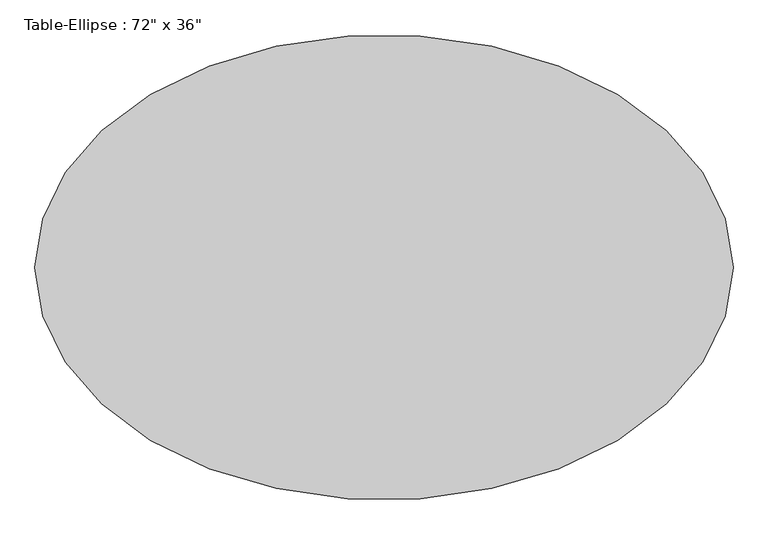
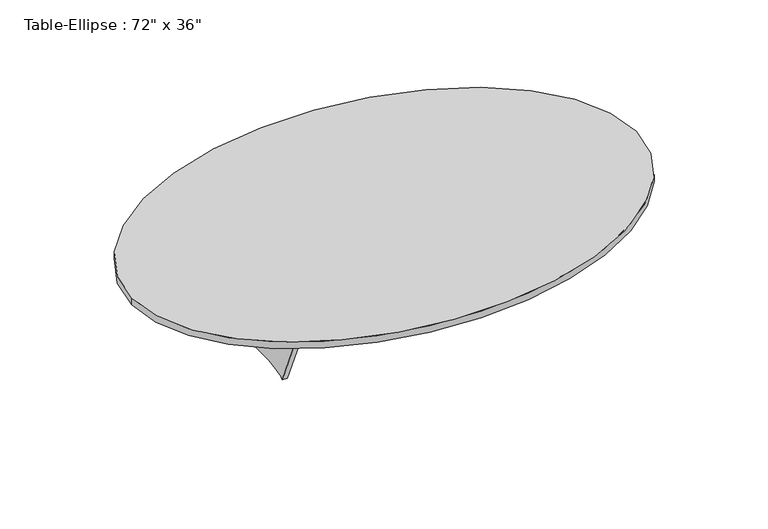
"""IFC4 building model written with IfcOpenShell, lengths in millimetres: furniture geometry."""

from ifc_helpers import new_model, si_unit, point, frame, origin, place, context, project, spatial, ellipse_curve, trimmed, source, transform, mapped, element, save
from ifc_brep_helpers import plane_surface, extruded_surface, advanced_brep


def furniture_1a6705e8(model_context):
    return source(origin(), model_context, "Body", "AdvancedBrep", [
        advanced_brep(
        [(-876.3, 19.05, 711.2), (876.3, 19.05, 711.2), (876.3, 19.05, 474.1333333), (-876.3, 19.05, 474.1333333), (-876.3, -19.05, 711.2), (-876.3, -19.05, 474.1333333), (876.3, -19.05, 474.1333333), (876.3, -19.05, 711.2)],
        [
            (0, 1),
            (1, 2),
            (2, 3, ellipse_curve(frame((0.0, 19.05, 474.1333333), z_axis=(0.0, -1.0, 0.0), x_axis=(1.0, 0.0, 0.0)), 876.3, 101.6)),
            (3, 0),
            (4, 5),
            (5, 6, ellipse_curve(frame((0.0, -19.05, 474.1333333), z_axis=(0.0, 1.0, 0.0), x_axis=(1.0, 0.0, 0.0)), 876.3, 101.6)),
            (6, 7),
            (7, 4),
            (0, 4),
            (7, 1),
            (6, 2),
            (5, 3),
        ],
        [
            plane_surface(frame((-876.3, 19.05, 711.2), z_axis=(0.0, 1.0, 0.0), x_axis=(1.0, 0.0, 0.0))),
            plane_surface(frame((-876.3, -19.05, 711.2), z_axis=(0.0, -1.0, 0.0), x_axis=(-1.0, 0.0, 0.0))),
            plane_surface(frame((-876.3, 19.05, 711.2), z_axis=(0.0, 0.0, 1.0), x_axis=(0.0, -1.0, 0.0))),
            plane_surface(frame((876.3, 19.05, 711.2), z_axis=(1.0, 0.0, 0.0), x_axis=(0.0, -1.0, 0.0))),
            extruded_surface(trimmed(ellipse_curve(frame((0.0, -57.15, 474.1333333), z_axis=(0.0, -1.0, 0.0), x_axis=(1.0, 0.0, 0.0)), 876.3, 101.6), [point((876.3, -57.15, 474.1333333))], [point((-876.3, -57.15, 474.1333333))], True, "CARTESIAN"), (0.0, 38.099999999999994, 0.0), 38.099999999999994),
            plane_surface(frame((-876.3, 19.05, 474.1333333), z_axis=(-1.0, 0.0, 0.0), x_axis=(0.0, -1.0, 0.0))),
        ],
        [
            (0, [[1, 2, 3, 4]]),
            (1, [[5, 6, 7, 8]]),
            (2, [[-1, 9, -8, 10]]),
            (3, [[-2, -10, -7, 11]]),
            (4, [[-3, -11, -6, 12]]),
            (5, [[-4, -12, -5, -9]]),
        ],
    ),
        advanced_brep(
        [(914.4, 609.6, 711.2), (914.4, -609.6, 711.2), (914.4, -304.8, 0.0), (914.4, 304.8, 0.0), (876.3, 609.6, 711.2), (876.3, 304.8, 0.0), (876.3, -304.8, 0.0), (876.3, -609.6, 711.2)],
        [
            (0, 1),
            (1, 2),
            (2, 3, ellipse_curve(frame((914.4, 0.0, 0.0), z_axis=(-1.0, 0.0, 0.0), x_axis=(0.0, 1.0, 0.0)), 304.8, 50.8)),
            (3, 0),
            (4, 5),
            (5, 6, ellipse_curve(frame((876.3, 0.0, 0.0), z_axis=(1.0, 0.0, 0.0), x_axis=(0.0, 1.0, 0.0)), 304.8, 50.8)),
            (6, 7),
            (7, 4),
            (0, 4),
            (7, 1),
            (6, 2),
            (5, 3),
        ],
        [
            plane_surface(frame((914.4, -609.6, 711.2), z_axis=(1.0, 0.0, 0.0), x_axis=(0.0, -1.0, 0.0))),
            plane_surface(frame((876.3, -609.6, 711.2), z_axis=(-1.0, 0.0, 0.0), x_axis=(0.0, 1.0, 0.0))),
            plane_surface(frame((914.4, 609.6, 711.2), z_axis=(0.0, 0.0, 1.0), x_axis=(-1.0, 0.0, 0.0))),
            plane_surface(frame((914.4, -609.6, 711.2), z_axis=(0.0, -0.919145030018057, -0.39391929857916985), x_axis=(-1.0, 0.0, 0.0))),
            extruded_surface(trimmed(ellipse_curve(frame((838.2, 0.0, 0.0), z_axis=(-1.0, 0.0, 0.0), x_axis=(0.0, 1.0, 0.0)), 304.8, 50.8), [point((838.2, -304.8, 0.0))], [point((838.2, 304.8, 0.0))], True, "CARTESIAN"), (38.09999999999991, 0.0, 0.0), 38.09999999999991),
            plane_surface(frame((914.4, 304.8, 0.0), z_axis=(0.0, 0.9191450300180644, -0.3939192985791526), x_axis=(-1.0, 0.0, 0.0))),
        ],
        [
            (0, [[1, 2, 3, 4]]),
            (1, [[5, 6, 7, 8]]),
            (2, [[-1, 9, -8, 10]]),
            (3, [[-2, -10, -7, 11]]),
            (4, [[-3, -11, -6, 12]]),
            (5, [[-4, -12, -5, -9]]),
        ],
    ),
        advanced_brep(
        [(-876.3, 609.6, 711.2), (-876.3, -609.6, 711.2), (-876.3, -304.8, 0.0), (-876.3, 304.8, 0.0), (-914.4, 609.6, 711.2), (-914.4, 304.8, 0.0), (-914.4, -304.8, 0.0), (-914.4, -609.6, 711.2)],
        [
            (0, 1),
            (1, 2),
            (2, 3, ellipse_curve(frame((-876.3, 0.0, 0.0), z_axis=(-1.0, 0.0, 0.0), x_axis=(0.0, 1.0, 0.0)), 304.8, 50.8)),
            (3, 0),
            (4, 5),
            (5, 6, ellipse_curve(frame((-914.4, 0.0, 0.0), z_axis=(1.0, 0.0, 0.0), x_axis=(0.0, 1.0, 0.0)), 304.8, 50.8)),
            (6, 7),
            (7, 4),
            (0, 4),
            (7, 1),
            (6, 2),
            (5, 3),
        ],
        [
            plane_surface(frame((-876.3, -609.6, 711.2), z_axis=(1.0, 0.0, 0.0), x_axis=(0.0, -1.0, 0.0))),
            plane_surface(frame((-914.4, -609.6, 711.2), z_axis=(-1.0, 0.0, 0.0), x_axis=(0.0, 1.0, 0.0))),
            plane_surface(frame((-876.3, 609.6, 711.2), z_axis=(0.0, 0.0, 1.0), x_axis=(-1.0, 0.0, 0.0))),
            plane_surface(frame((-876.3, -609.6, 711.2), z_axis=(0.0, -0.919145030018057, -0.3939192985791699), x_axis=(-1.0, 0.0, 0.0))),
            extruded_surface(trimmed(ellipse_curve(frame((-952.5, 0.0, 0.0), z_axis=(-1.0, 0.0, 0.0), x_axis=(0.0, 1.0, 0.0)), 304.8, 50.8), [point((-952.5, -304.8, 0.0))], [point((-952.5, 304.8, 0.0))], True, "CARTESIAN"), (38.10000000000002, 0.0, 0.0), 38.10000000000002),
            plane_surface(frame((-876.3, 304.8, 0.0), z_axis=(0.0, 0.9191450300180607, -0.3939192985791611), x_axis=(-1.0, 0.0, 0.0))),
        ],
        [
            (0, [[1, 2, 3, 4]]),
            (1, [[5, 6, 7, 8]]),
            (2, [[-1, 9, -8, 10]]),
            (3, [[-2, -10, -7, 11]]),
            (4, [[-3, -11, -6, 12]]),
            (5, [[-4, -12, -5, -9]]),
        ],
    ),
        advanced_brep(
        [(-1828.8, 0.0, 762.0), (1828.8, 0.0, 762.0), (-1828.8, 0.0, 711.2), (1828.8, 0.0, 711.2)],
        [
            (0, 1, ellipse_curve(frame((0.0, 0.0, 762.0), z_axis=(0.0, 0.0, 1.0), x_axis=(1.0, 0.0, 0.0)), 1828.8, 1219.2)),
            (1, 0, ellipse_curve(frame((0.0, 0.0, 762.0), z_axis=(0.0, 0.0, 1.0), x_axis=(1.0, 0.0, 0.0)), 1828.8, 1219.2)),
            (2, 3, ellipse_curve(frame((0.0, 0.0, 711.2), z_axis=(0.0, 0.0, -1.0), x_axis=(1.0, 0.0, 0.0)), 1828.8, 1219.2)),
            (3, 2, ellipse_curve(frame((0.0, 0.0, 711.2), z_axis=(0.0, 0.0, -1.0), x_axis=(1.0, 0.0, 0.0)), 1828.8, 1219.2)),
            (0, 2),
            (3, 1),
        ],
        [
            plane_surface(frame((1828.8, 0.0, 762.0), z_axis=(0.0, 0.0, 1.0), x_axis=(0.0, 1.0, 0.0))),
            plane_surface(frame((1828.8, 0.0, 711.2), z_axis=(0.0, 0.0, -1.0), x_axis=(0.0, -1.0, 0.0))),
            extruded_surface(trimmed(ellipse_curve(frame((0.0, 0.0, 660.4), z_axis=(0.0, 0.0, 1.0), x_axis=(1.0, 0.0, 0.0)), 1828.8, 1219.2), [point((-1828.8, 0.0, 660.4))], [point((1828.8, 0.0, 660.4))], True, "CARTESIAN"), (0.0, 0.0, 50.80000000000007), 50.80000000000007),
            extruded_surface(trimmed(ellipse_curve(frame((0.0, 0.0, 660.4), z_axis=(0.0, 0.0, 1.0), x_axis=(1.0, 0.0, 0.0)), 1828.8, 1219.2), [point((1828.8, 0.0, 660.4))], [point((-1828.8, 0.0, 660.4))], True, "CARTESIAN"), (0.0, 0.0, 50.80000000000007), 50.80000000000007),
        ],
        [
            (0, [[1, 2]]),
            (1, [[3, 4]]),
            (2, [[-1, 5, -4, 6]]),
            (3, [[-2, -6, -3, -5]]),
        ],
    ),
    ])


if __name__ == "__main__":
    model = new_model("IFC4")
    model_context = context("Model", 3, world=origin())
    ifc_project = project(units=[si_unit("LENGTHUNIT", "METRE", prefix="MILLI")], contexts=[model_context])
    site = spatial("IfcSite", under=ifc_project)
    building = spatial("IfcBuilding", under=site)
    placement = place(None, origin())
    furniture_shape = furniture_1a6705e8(model_context)
    element("IfcFurniture", 1, ObjectType="Table-Ellipse : 72\" x 36\"", at=placement, inside=building, context=model_context, shape_type="MappedRepresentation", body=[
        mapped(furniture_shape, transform((0.0, 0.0, 0.0), x_axis=(1.0, 0.0, 0.0), y_axis=(0.0, 1.0, 0.0), z_axis=(0.0, 0.0, 1.0))),
    ])
    save(model, "model.ifc")

# Revit data of these elements
# Type "Table-Ellipse : 72\" x 36\""
#   Assembly Code = "E2020200"
#   Half Width = 4' - 0"
#   Half Length = 6' - 0"
#   Height = 2' - 6"
#   Length = 12' - 0"
#   Width = 8' - 0"
#   Base Material = Birch
#   Top Material = Laminate - Black
#   Default Elevation = 0
# Element 1 (IfcFurniture, "Table-Ellipse : 72\" x 36\"")
#   Materials on its faces: "Birch", "Laminate - Black"
# Materials
#   "Birch": class "Wood", colour RGB 224 178 126, transparency 0, Description = "Betula Alleghaniensis", Cost = 0
#   "Laminate - Black": colour RGB 0 0 0, transparency 0
